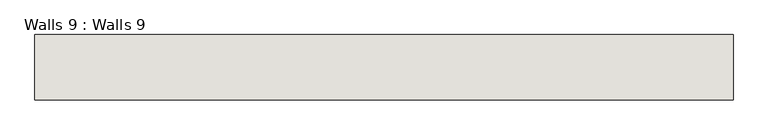
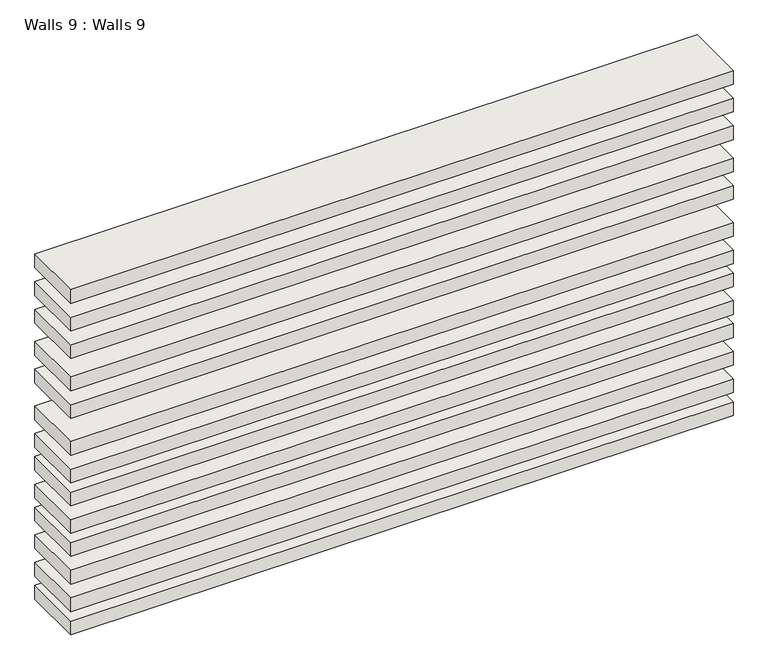
"""IFC4 building model written with IfcOpenShell, lengths in millimetres: wall geometry, Walls 9 : Walls 9."""

from ifc_helpers import new_model, si_unit, frame, origin, place, context, project, spatial, polyline, outline, extrude, source, transform, mapped, element, save


def walls_9_walls_9_57911b2c(model_context):
    return source(origin(), model_context, "Body", "SweptSolid", [
        extrude(outline(polyline([(-3427.5361288, -17646.2071125), (-6881.9361288, -17646.2071125), (-6881.9361288, -17322.090882), (-3427.5361288, -17322.090882), (-3427.5361288, -17646.2071125)])), frame((0.0, 0.0, 50.0), z_axis=(0.0, 0.0, 1.0), x_axis=(1.0, 0.0, 0.0)), (0.0, 0.0, 1.0), 75.9070443),
        extrude(outline(polyline([(-3427.5361288, -17646.2071125), (-6881.9361288, -17646.2071125), (-6881.9361288, -17322.090882), (-3427.5361288, -17322.090882), (-3427.5361288, -17646.2071125)])), frame((0.0, 0.0, 177.0), z_axis=(0.0, 0.0, 1.0), x_axis=(1.0, 0.0, 0.0)), (0.0, 0.0, 1.0), 75.9070443),
        extrude(outline(polyline([(-3427.5361288, -17646.2071125), (-6881.9361288, -17646.2071125), (-6881.9361288, -17322.090882), (-3427.5361288, -17322.090882), (-3427.5361288, -17646.2071125)])), frame((0.0, 0.0, 329.4), z_axis=(0.0, 0.0, 1.0), x_axis=(1.0, 0.0, 0.0)), (0.0, 0.0, 1.0), 75.9070443),
        extrude(outline(polyline([(-3427.5361288, -17646.2071125), (-6881.9361288, -17646.2071125), (-6881.9361288, -17322.090882), (-3427.5361288, -17322.090882), (-3427.5361288, -17646.2071125)])), frame((0.0, 0.0, 481.8), z_axis=(0.0, 0.0, 1.0), x_axis=(1.0, 0.0, 0.0)), (0.0, 0.0, 1.0), 75.9070443),
        extrude(outline(polyline([(-3427.5361288, -17646.2071125), (-6881.9361288, -17646.2071125), (-6881.9361288, -17322.090882), (-3427.5361288, -17322.090882), (-3427.5361288, -17646.2071125)])), frame((0.0, 0.0, 608.8), z_axis=(0.0, 0.0, 1.0), x_axis=(1.0, 0.0, 0.0)), (0.0, 0.0, 1.0), 75.9070443),
        extrude(outline(polyline([(-3427.5361288, -17646.2071125), (-6881.9361288, -17646.2071125), (-6881.9361288, -17322.090882), (-3427.5361288, -17322.090882), (-3427.5361288, -17646.2071125)])), frame((0.0, 0.0, 761.2), z_axis=(0.0, 0.0, 1.0), x_axis=(1.0, 0.0, 0.0)), (0.0, 0.0, 1.0), 75.9070443),
        extrude(outline(polyline([(-3427.5361288, -17646.2071125), (-6881.9361288, -17646.2071125), (-6881.9361288, -17322.090882), (-3427.5361288, -17322.090882), (-3427.5361288, -17646.2071125)])), frame((0.0, 0.0, 888.2), z_axis=(0.0, 0.0, 1.0), x_axis=(1.0, 0.0, 0.0)), (0.0, 0.0, 1.0), 75.9070443),
        extrude(outline(polyline([(-3427.5361288, -17646.2071125), (-6881.9361288, -17646.2071125), (-6881.9361288, -17322.090882), (-3427.5361288, -17322.090882), (-3427.5361288, -17646.2071125)])), frame((0.0, 0.0, 1040.6), z_axis=(0.0, 0.0, 1.0), x_axis=(1.0, 0.0, 0.0)), (0.0, 0.0, 1.0), 75.9070443),
        extrude(outline(polyline([(-3427.5361288, -17646.2071125), (-6881.9361288, -17646.2071125), (-6881.9361288, -17322.090882), (-3427.5361288, -17322.090882), (-3427.5361288, -17646.2071125)])), frame((0.0, 0.0, 1243.8), z_axis=(0.0, 0.0, 1.0), x_axis=(1.0, 0.0, 0.0)), (0.0, 0.0, 1.0), 75.9070443),
        extrude(outline(polyline([(-3427.5361288, -17646.2071125), (-6881.9361288, -17646.2071125), (-6881.9361288, -17322.090882), (-3427.5361288, -17322.090882), (-3427.5361288, -17646.2071125)])), frame((0.0, 0.0, 1396.2), z_axis=(0.0, 0.0, 1.0), x_axis=(1.0, 0.0, 0.0)), (0.0, 0.0, 1.0), 75.9070443),
        extrude(outline(polyline([(-3427.5361288, -17646.2071125), (-6881.9361288, -17646.2071125), (-6881.9361288, -17322.090882), (-3427.5361288, -17322.090882), (-3427.5361288, -17646.2071125)])), frame((0.0, 0.0, 1574.0), z_axis=(0.0, 0.0, 1.0), x_axis=(1.0, 0.0, 0.0)), (0.0, 0.0, 1.0), 75.9070443),
        extrude(outline(polyline([(-3427.5361288, -17646.2071125), (-6881.9361288, -17646.2071125), (-6881.9361288, -17322.090882), (-3427.5361288, -17322.090882), (-3427.5361288, -17646.2071125)])), frame((0.0, 0.0, 1726.4), z_axis=(0.0, 0.0, 1.0), x_axis=(1.0, 0.0, 0.0)), (0.0, 0.0, 1.0), 75.9070443),
        extrude(outline(polyline([(-3427.5361288, -17646.2071125), (-6881.9361288, -17646.2071125), (-6881.9361288, -17322.090882), (-3427.5361288, -17322.090882), (-3427.5361288, -17646.2071125)])), frame((0.0, 0.0, 1878.8), z_axis=(0.0, 0.0, 1.0), x_axis=(1.0, 0.0, 0.0)), (0.0, 0.0, 1.0), 75.9070443),
    ])


if __name__ == "__main__":
    model = new_model("IFC4")
    model_context = context("Model", 3, world=origin())
    ifc_project = project(units=[si_unit("LENGTHUNIT", "METRE", prefix="MILLI")], contexts=[model_context])
    site = spatial("IfcSite", under=ifc_project)
    building = spatial("IfcBuilding", under=site)
    placement = place(None, origin())
    walls_9_walls_9_shape = walls_9_walls_9_57911b2c(model_context)
    element("IfcWall", 1, ObjectType="Walls 9 : Walls 9", at=placement, inside=building, context=model_context, shape_type="MappedRepresentation", body=[
        mapped(walls_9_walls_9_shape, transform((0.0, 0.0, 0.0), x_axis=(1.0, 0.0, 0.0), y_axis=(0.0, 1.0, 0.0), z_axis=(0.0, 0.0, 1.0))),
    ])
    save(model, "model.ifc")

# Revit data of these elements
# Element 1 (IfcWall, "Walls 9 : Walls 9")
#   Materials on its faces: "Default Wall", "Door - Frame"
# Materials
#   "Default Wall": colour RGB 128 128 128, transparency 0
#   "Door - Frame": colour RGB 118 70 51, transparency 0
